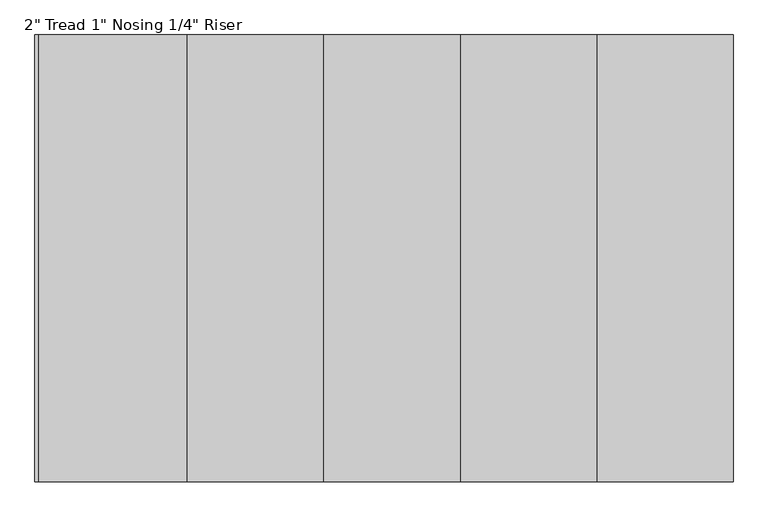
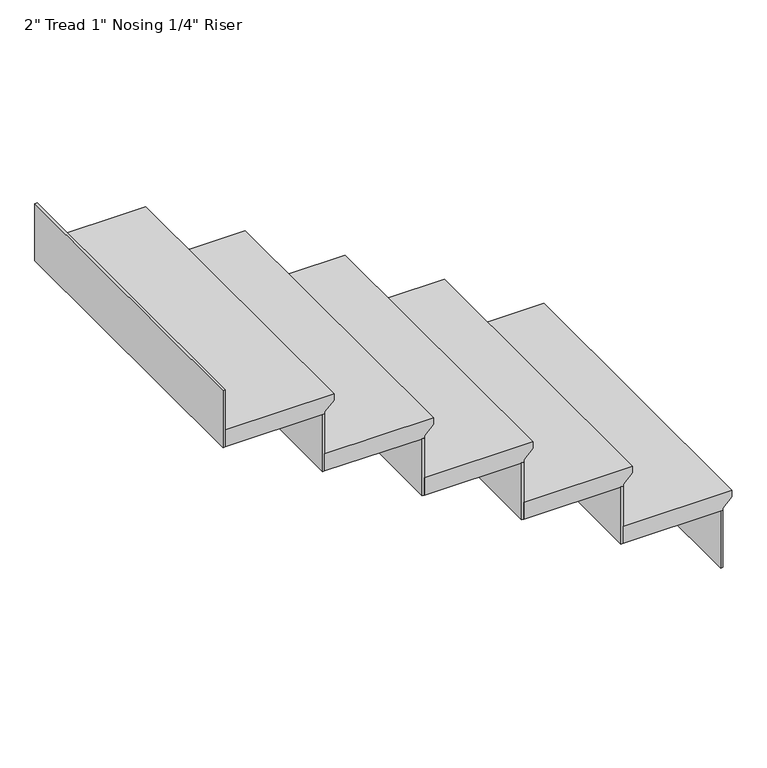
"""IFC4 building model written with IfcOpenShell, lengths in millimetres: stair flight geometry."""

from ifc_helpers import new_model, si_unit, frame, origin, place, context, project, spatial, polyline, outline, extrude, source, transform, mapped, element, save


def stair_flight_74d64587(model_context):
    return source(origin(), model_context, "Body", "SweptSolid", [
        extrude(outline(polyline([(2709.3333333, -43.108395), (2709.3333333, -347.908395), (2658.5333333, -347.908395), (2658.5333333, -68.508395), (2664.8833333, -68.508395), (2690.2833333, -43.108395), (2709.3333333, -43.108395)])), frame((0.0, -1569.3848818, 0.0), z_axis=(0.0, 1.0, 0.0), x_axis=(0.0, 0.0, 1.0)), (0.0, 0.0, 1.0), 914.4),
        extrude(outline(polyline([(-74.858395, -654.9848818), (-68.508395, -654.9848818), (-68.508395, -1569.3848818), (-74.858395, -1569.3848818), (-74.858395, -654.9848818)])), frame((0.0, 0.0, 2489.2), z_axis=(0.0, 0.0, 1.0), x_axis=(1.0, 0.0, 0.0)), (0.0, 0.0, 1.0), 169.3333333),
        extrude(outline(polyline([(-354.258395, -654.9848818), (-347.908395, -654.9848818), (-347.908395, -1569.3848818), (-354.258395, -1569.3848818), (-354.258395, -654.9848818)])), frame((0.0, 0.0, 2658.5333333), z_axis=(0.0, 0.0, 1.0), x_axis=(1.0, 0.0, 0.0)), (0.0, 0.0, 1.0), 169.3333333),
        extrude(outline(polyline([(2878.6666667, -322.508395), (2878.6666667, -627.308395), (2827.8666667, -627.308395), (2827.8666667, -347.908395), (2834.2166667, -347.908395), (2859.6166667, -322.508395), (2878.6666667, -322.508395)])), frame((0.0, -1569.3848818, 0.0), z_axis=(0.0, 1.0, 0.0), x_axis=(0.0, 0.0, 1.0)), (0.0, 0.0, 1.0), 914.4),
        extrude(outline(polyline([(-633.658395, -654.9848818), (-627.308395, -654.9848818), (-627.308395, -1569.3848818), (-633.658395, -1569.3848818), (-633.658395, -654.9848818)])), frame((0.0, 0.0, 2827.8666667), z_axis=(0.0, 0.0, 1.0), x_axis=(1.0, 0.0, 0.0)), (0.0, 0.0, 1.0), 169.3333333),
        extrude(outline(polyline([(3048.0, -601.908395), (3048.0, -906.708395), (2997.2, -906.708395), (2997.2, -627.308395), (3003.55, -627.308395), (3028.95, -601.908395), (3048.0, -601.908395)])), frame((0.0, -1569.3848818, 0.0), z_axis=(0.0, 1.0, 0.0), x_axis=(0.0, 0.0, 1.0)), (0.0, 0.0, 1.0), 914.4),
        extrude(outline(polyline([(-913.058395, -654.9848818), (-906.708395, -654.9848818), (-906.708395, -1569.3848818), (-913.058395, -1569.3848818), (-913.058395, -654.9848818)])), frame((0.0, 0.0, 2997.2), z_axis=(0.0, 0.0, 1.0), x_axis=(1.0, 0.0, 0.0)), (0.0, 0.0, 1.0), 169.3333333),
        extrude(outline(polyline([(3217.3333333, -881.308395), (3217.3333333, -1186.108395), (3166.5333333, -1186.108395), (3166.5333333, -906.708395), (3172.8833333, -906.708395), (3198.2833333, -881.308395), (3217.3333333, -881.308395)])), frame((0.0, -1569.3848818, 0.0), z_axis=(0.0, 1.0, 0.0), x_axis=(0.0, 0.0, 1.0)), (0.0, 0.0, 1.0), 914.4),
        extrude(outline(polyline([(-1192.458395, -654.9848818), (-1186.108395, -654.9848818), (-1186.108395, -1569.3848818), (-1192.458395, -1569.3848818), (-1192.458395, -654.9848818)])), frame((0.0, 0.0, 3166.5333333), z_axis=(0.0, 0.0, 1.0), x_axis=(1.0, 0.0, 0.0)), (0.0, 0.0, 1.0), 169.3333333),
        extrude(outline(polyline([(-1471.858395, -654.9848818), (-1465.508395, -654.9848818), (-1465.508395, -1569.3848818), (-1471.858395, -1569.3848818), (-1471.858395, -654.9848818)])), frame((0.0, 0.0, 3335.8666667), z_axis=(0.0, 0.0, 1.0), x_axis=(1.0, 0.0, 0.0)), (0.0, 0.0, 1.0), 169.3333333),
        extrude(outline(polyline([(3386.6666667, -1160.708395), (3386.6666667, -1465.508395), (3335.8666667, -1465.508395), (3335.8666667, -1186.108395), (3342.2166667, -1186.108395), (3367.6166667, -1160.708395), (3386.6666667, -1160.708395)])), frame((0.0, -1569.3848818, 0.0), z_axis=(0.0, 1.0, 0.0), x_axis=(0.0, 0.0, 1.0)), (0.0, 0.0, 1.0), 914.4),
    ])


if __name__ == "__main__":
    model = new_model("IFC4")
    model_context = context("Model", 3, world=origin())
    ifc_project = project(units=[si_unit("LENGTHUNIT", "METRE", prefix="MILLI")], contexts=[model_context])
    site = spatial("IfcSite", under=ifc_project)
    building = spatial("IfcBuilding", under=site)
    placement = place(None, origin())
    stair_flight_shape = stair_flight_74d64587(model_context)
    element("IfcStairFlight", 1, ObjectType="2\" Tread 1\" Nosing 1/4\" Riser", at=placement, inside=building, context=model_context, shape_type="MappedRepresentation", body=[
        mapped(stair_flight_shape, transform((0.0, 0.0, 0.0), x_axis=(1.0, 0.0, 0.0), y_axis=(0.0, 1.0, 0.0), z_axis=(0.0, 0.0, 1.0))),
    ])
    save(model, "model.ifc")
